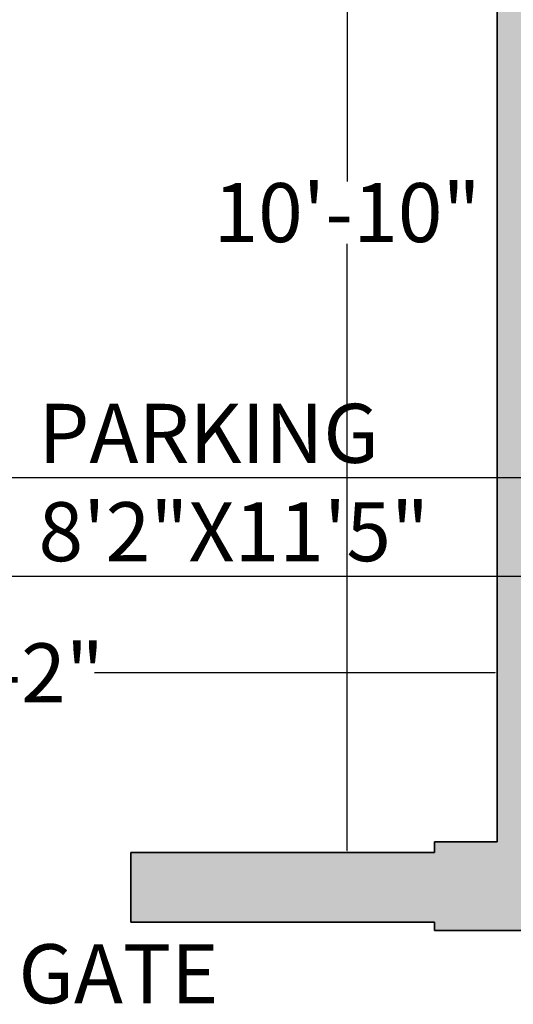
# Model space of a CAD drawing. Units: inches. Extents: x -5 to 482, y -460 to 66.
# Tile 8 of 31: x 91 to 142, y -429 to -329. Entities that reach past the tile are written whole.
import ezdxf

# ---------------------------------------------------------------- set-up
doc = ezdxf.new("R2010")
doc.units = ezdxf.units.IN
doc.header["$MEASUREMENT"] = 0
for name, color, linetype, lineweight in [('A-ANNO-DIMS', 2, 'Continuous', 18), ('A-ANNO-TEXT', 7, 'Continuous', 18), ('A-AREA-IDEN', 7, 'Continuous', 18), ('A-WALL', 7, 'Continuous', 35), ('A-WALL-PATT', 152, 'Continuous', 13)]:
    doc.layers.add(name, color=color, linetype=linetype, lineweight=lineweight)
doc.styles.get("Standard").update_dxf_attribs({"font": 'arial.ttf'})
doc.dimstyles.get("Standard").update_dxf_attribs({"dimtxt": 0.18, "dimasz": 0.18, "dimexe": 0.18, "dimexo": 0.0625, "dimgap": 0.09, "dimtad": 0, "dimtih": 1, "dimtoh": 1, "dimdec": 0, "dimzin": 0, "dimdsep": 46, "dimlunit": 3, "dimtxsty": 'Standard', "dimcen": 0.09, "dimadec": 0, "dimazin": 0, "dimtfac": 1, "dimtdec": 0, "dimtofl": 0, "dimtmove": 0, "dimatfit": 3, "dimfxl": 1, "dimtolj": 1, "dimtzin": 0, "dimarcsym": 0})

# ---------------------------------------------------------------- blocks, each defined once
blk = doc.blocks.new('*D21')
at = {"layer": 'A-ANNO-DIMS', "color": 0, "lineweight": -2, "transparency": 16777216}
for p, q in [((133.45, -283.85), (124.45, -283.85)), ((124.63, -284.03), (124.63, -345.73)), ((124.63, -413.74), (124.63, -352.04)), ((124.69, -413.92), (124.81, -413.92))]:
    blk.add_line(p, q, dxfattribs=at)
at = {"layer": 'A-ANNO-DIMS', "color": 0, "transparency": 16777216}
for points in [[(124.6, -284.03), (124.66, -284.03), (124.63, -283.85)], [(124.6, -413.74), (124.66, -413.74), (124.63, -413.92)]]:
    blk.add_solid(points, dxfattribs=at)
at = {"layer": 'Defpoints', "color": 0, "transparency": 16777216}
for p in [(124.63, -283.85), (133.51, -283.85), (124.63, -413.92)]:
    blk.add_point(p, dxfattribs=at)
at = {"layer": 'A-ANNO-DIMS', "color": 0, "transparency": 16777216, "insert": (124.63, -348.88), "char_height": 6, "attachment_point": 5}
blk.add_mtext('\\A1;10\'-10"', dxfattribs=at)
blk = doc.blocks.new('*D22')
at = {"layer": 'A-ANNO-DIMS', "color": 0, "lineweight": -2, "transparency": 16777216}
for p, q in [((41.88, -395.6), (41.88, -395.49)), ((42.06, -395.67), (82.81, -395.67)), ((139.7, -395.67), (98.95, -395.67)), ((139.88, -395.6), (139.88, -395.49))]:
    blk.add_line(p, q, dxfattribs=at)
at = {"layer": 'A-ANNO-DIMS', "color": 0, "transparency": 16777216}
for points in [[(42.06, -395.64), (42.06, -395.7), (41.88, -395.67)], [(139.7, -395.64), (139.7, -395.7), (139.88, -395.67)]]:
    blk.add_solid(points, dxfattribs=at)
at = {"layer": 'Defpoints', "color": 0, "transparency": 16777216}
for p in [(41.88, -395.67), (139.88, -395.67), (139.88, -395.67)]:
    blk.add_point(p, dxfattribs=at)
at = {"layer": 'A-ANNO-DIMS', "color": 0, "transparency": 16777216, "insert": (90.88, -395.67), "char_height": 6, "attachment_point": 5}
blk.add_mtext('\\A1;8\'-2"', dxfattribs=at)
blk = doc.blocks.new('*D72')
at = {"layer": 'A-ANNO-DIMS', "color": 0, "lineweight": -2, "transparency": 16777216}
for p, q in [((144.31, -375.86), (-4.9, -375.86)), ((-4.72, -376.04), (-4.72, -380.68)), ((-4.72, -385.68), (-4.72, -381.04)), ((144.31, -385.86), (-4.9, -385.86))]:
    blk.add_line(p, q, dxfattribs=at)
at = {"layer": 'A-ANNO-DIMS', "color": 0, "transparency": 16777216}
for points in [[(-4.75, -376.04), (-4.69, -376.04), (-4.72, -375.86)], [(-4.75, -385.68), (-4.69, -385.68), (-4.72, -385.86)]]:
    blk.add_solid(points, dxfattribs=at)
at = {"layer": 'Defpoints', "color": 0, "transparency": 16777216}
for p in [(144.38, -375.86), (-4.72, -385.86), (144.38, -385.86)]:
    blk.add_point(p, dxfattribs=at)
at = {"layer": 'A-ANNO-DIMS', "color": 0, "transparency": 16777216, "insert": (-4.72, -380.86), "char_height": 0.18, "attachment_point": 5}
blk.add_mtext('\\A1;0\'-10"', dxfattribs=at)

msp = doc.modelspace()

# ---------------------------------------------------------------- hatches: boundary and pattern name
at = {"layer": 'A-WALL-PATT'}
h = msp.add_hatch(color=256, dxfattribs=at)
h.dxf.hatch_style = 1
h.paths.add_polyline_path([(149.38, -412.85), (144.38, -412.85), (144.38, -283.85), (144.38, -279.35), (133.88, -279.35), (133.88, -283.85), (139.88, -283.85), (139.88, -412.85), (133.51, -412.85), (133.51, -413.92), (102.65, -413.92), (102.65, -421.02), (133.51, -421.02), (133.51, -421.85), (149.38, -421.85)])
h.paths.add_polyline_path([(226.05, -412.85), (218.88, -412.85), (218.88, -350.85), (262.88, -350.85), (262.88, -386.85), (267.38, -386.85), (267.38, -283.85), (270.38, -283.85), (270.38, -279.35), (244.88, -279.35), (244.88, -283.85), (262.88, -283.85), (262.88, -346.35), (218.88, -346.35), (218.88, -283.85), (220.88, -283.85), (220.88, -279.35), (214.38, -279.35), (214.38, -283.85), (214.38, -412.85), (209.38, -412.85), (209.38, -421.85), (226.05, -421.85)])
h.paths.add_polyline_path([(315.81, -412.85), (250.05, -412.85), (250.05, -421.85), (315.81, -421.85)])
h.paths.add_polyline_path([(430.38, -378.35), (421.38, -378.35), (421.38, -412.85), (375.81, -412.85), (375.81, -421.85), (430.38, -421.85)])
h.paths.add_polyline_path([(78.69, -413.92), (47.68, -413.92), (47.68, -412.85), (41.88, -412.85), (41.88, -283.85), (109.88, -283.85), (109.88, -279.35), (41.88, -279.35), (41.88, -241.85), (32.88, -241.85), (32.88, -421.85), (47.68, -421.85), (47.68, -421.02), (78.69, -421.02)])
h.paths.add_polyline_path([(41.88, -144.35), (154.38, -144.35), (154.38, -137.85), (149.88, -137.85), (149.88, -139.85), (41.88, -139.85), (41.88, -97.85), (32.88, -97.85), (32.88, -181.85), (41.88, -181.85)])
h.paths.add_polyline_path([(430.38, -241.85), (421.38, -241.85), (421.38, -279.35), (309.38, -279.35), (309.38, -170.35), (304.88, -170.35), (304.88, -279.35), (294.38, -279.35), (294.38, -283.85), (421.38, -283.85), (421.38, -318.35), (430.38, -318.35)])
h.paths.add_polyline_path([(430.38, -119.85), (421.38, -119.85), (421.38, -139.85), (419.38, -139.85), (419.38, -144.35), (421.38, -144.35), (421.38, -181.85), (430.38, -181.85)])
h.paths.add_polyline_path([(395.38, -139.85), (377.38, -139.85), (377.38, -75.85), (421.38, -75.85), (421.38, -95.85), (430.38, -95.85), (430.38, -45.6), (421.38, -45.6), (421.38, -71.35), (377.38, -71.35), (377.38, -22.85), (372.88, -22.85), (372.88, -139.85), (242.88, -139.85), (242.88, -137.85), (238.38, -137.85), (238.38, -144.35), (304.88, -144.35), (304.88, -146.35), (309.38, -146.35), (309.38, -144.35), (395.38, -144.35)])
h.paths.add_polyline_path([(65.88, 13.15), (32.88, 13.15), (32.88, -37.85), (41.88, -37.85), (41.88, 4.15), (65.88, 4.15)])
h.paths.add_polyline_path([(166.38, 13.15), (125.88, 13.15), (125.88, 4.15), (149.88, 4.15), (149.88, -113.85), (154.38, -113.85), (154.38, 4.15), (166.38, 4.15)])
h.paths.add_polyline_path([(277.88, 13.15), (226.38, 13.15), (226.38, 4.15), (238.38, 4.15), (238.38, -113.85), (242.88, -113.85), (242.88, 4.15), (277.88, 4.15)])
h.paths.add_polyline_path([(430.38, 13.15), (337.88, 13.15), (337.88, 4.15), (372.88, 4.15), (372.88, 1.15), (377.38, 1.15), (377.38, 4.15), (421.38, 4.15), (421.38, -21.6), (430.38, -21.6)])

# ---------------------------------------------------------------- linework, layer by layer
at = {"layer": 'A-WALL'}
for p, q in [((139.88, -283.85), (139.88, -412.85)), ((133.51, -412.85), (133.51, -413.92)), ((133.51, -412.85), (139.88, -412.85)), ((133.51, -413.92), (102.65, -413.92)), ((102.65, -413.92), (102.65, -421.02)), ((133.51, -421.02), (102.65, -421.02)), ((133.51, -421.02), (133.51, -421.85)), ((133.51, -421.85), (430.38, -421.85))]:
    msp.add_line(p, q, dxfattribs=at)

# ---------------------------------------------------------------- texts
at = {"layer": 'A-ANNO-TEXT', "insert": (69.45, -423.26), "char_height": 6, "attachment_point": 1}
msp.add_mtext('MAIN GATE', dxfattribs=at)
at = {"layer": 'A-AREA-IDEN', "insert": (93.26, -368.32), "char_height": 6, "attachment_point": 1}
msp.add_mtext('PARKING\\P8\'2"X11\'5"', dxfattribs=at)

# ---------------------------------------------------------------- dimensions: what is measured, and where the dimension line sits
at = {"layer": 'A-ANNO-DIMS'}
for base, p1, p2, override, picture, middle in [((124.63, -283.85), (124.63, -413.92), (133.51, -283.85), {"dimtxt": 6, "dimclrd": 0, "dimclre": 0, "dimclrt": 0}, '*D21', (124.63, -348.88)), ((-4.72, -385.86), (144.38, -375.86), (144.38, -385.86), {"dimdec": 1, "dimlfac": 1, "dimrnd": 0, "dimzin": 1, "dimdsep": 46, "dimlunit": 4, "dimfrac": 2}, '*D72', (-4.72, -380.86))]:
    dim = msp.add_linear_dim(base=base, p1=p1, p2=p2, angle=90, dimstyle='Standard', override=override, dxfattribs=at)
    dim.commit()
    dim.dimension.update_dxf_attribs({"geometry": picture, "text_midpoint": middle})
dim = msp.add_linear_dim(base=(139.88, -395.67), p1=(41.88, -395.67), p2=(139.88, -395.67), dimstyle='Standard', override={"dimtxt": 6, "dimclrd": 0, "dimclre": 0, "dimclrt": 0}, dxfattribs=at)
dim.commit()
dim.dimension.update_dxf_attribs({"geometry": '*D22', "text_midpoint": (90.88, -395.67)})

doc.saveas('drawing.dxf')
